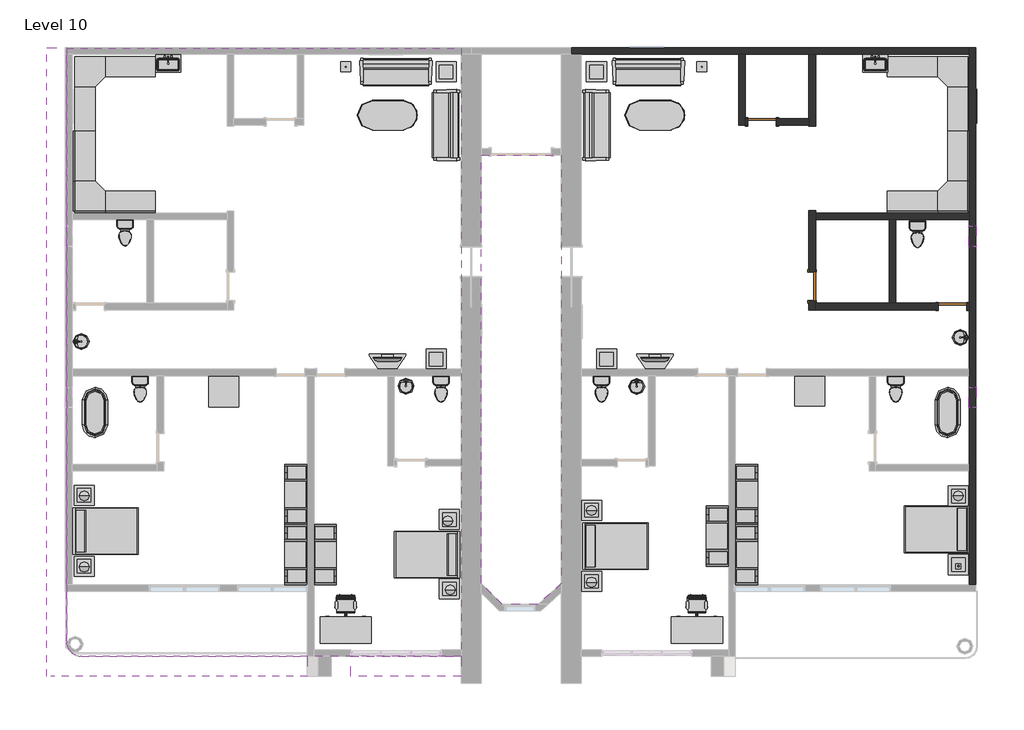
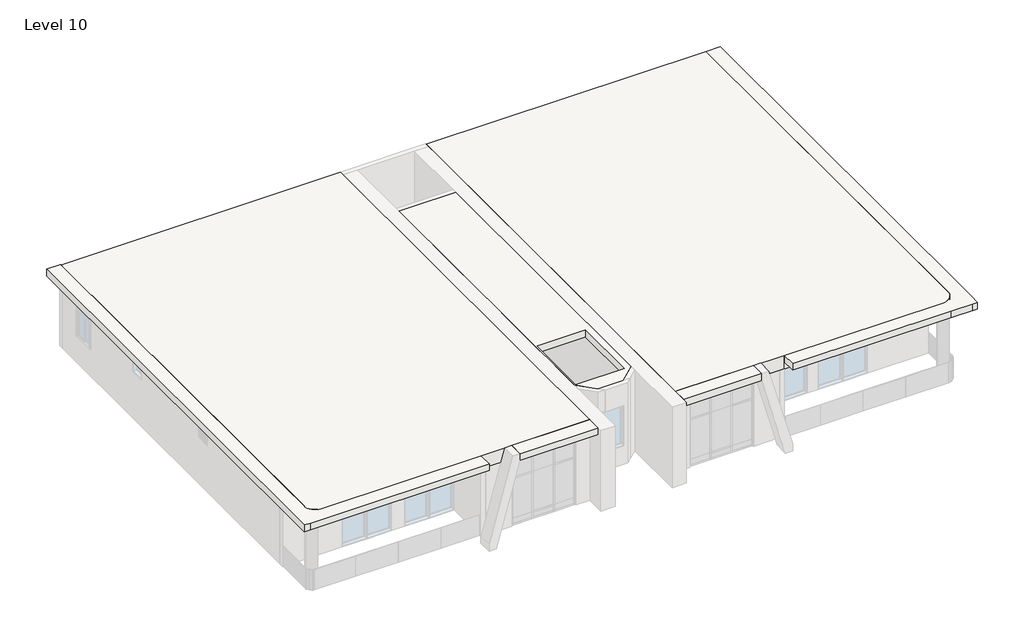
# One storey, part 3 of 3: 42 furniture elements, 14 flow terminals, 10 light fixtures, 9 walls, 4 slabs, 3 doors, 3 windows.
"""IFC4 building model written with IfcOpenShell, lengths in millimetres."""

from ifc_helpers import new_model, si_unit, point, frame, frame_2d, origin, place, context, project, spatial, polyline, circle_curve, trimmed, segment, composite_curve, outline, extrude, faceted_brep, transform, mapped, element, save
from components import door_2703ae13, door_10fd3a06, flow_terminal_38af2918, flow_terminal_d49f872f, toilet_domestic_3d_toilet_domestic_3d_f7549cf7, toilet_domestic_3d_toilet_domestic_3d_183bbd19, flow_terminal_b374fae2, furniture_07436f11, furniture_096e7f55, chair_task_arms_chair_task_arms_fa5a08ef, furniture_072f6425, furniture_cf0b6580, furniture_aff9b2fb, furniture_56245f3a, tv_stand_tv_stand_6ce107e5, furniture_b5c51a22, furniture_2c34a4f9, furniture_4d44e21c, furniture_45e3acac, light_fixture_100w_120v_8564026f, table_lamp_hemispheric_60w_120v_02721d88, window_0038ecf3, window_54100e87

model = new_model("IFC4")

# Units and contexts
model_context = context("Model", 3, world=origin())
ifc_project = project(units=[si_unit("LENGTHUNIT", "METRE", prefix="MILLI")], contexts=[model_context])

# Site, building, storey
site = spatial("IfcSite", under=ifc_project)
building = spatial("IfcBuilding", under=site)
storey = spatial("IfcBuildingStorey", under=building, Name="Level 10", Elevation=32918.4)

# Doors
placement = place(None, origin())
door_shape = door_2703ae13(model_context)
element("IfcDoor", 1, ObjectType="Door-Single-Panel.0001 : 34\" x 80\"", at=placement, inside=storey, context=model_context, shape_type="MappedRepresentation", body=[
    mapped(door_shape, transform((2522.0012296, 9464.0758558, 32918.4), x_axis=(-1.0, 0.0, 0.0), y_axis=(0.0, -1.0, 0.0), z_axis=(0.0, 0.0, 1.0))),
])
door_2_shape = door_10fd3a06(model_context)
element("IfcDoor", 2, ObjectType="Door-Single-Panel.0001 : 34\" x 80\"", at=placement, inside=storey, context=model_context, shape_type="MappedRepresentation", body=[
    mapped(door_2_shape, transform((8313.2012296, 3850.6758558, 32918.4), x_axis=(1.0, 0.0, 0.0), y_axis=(0.0, 1.0, 0.0), z_axis=(0.0, 0.0, 1.0))),
])
element("IfcDoor", 3, ObjectType="Door-Single-Panel.0001 : 34\" x 80\"", at=placement, inside=storey, context=model_context, shape_type="MappedRepresentation", body=[
    mapped(door_2_shape, transform((4046.0012296, 4460.2758558, 32918.4), x_axis=(0.0, -1.0, 0.0), y_axis=(1.0, 0.0, 0.0), z_axis=(0.0, 0.0, 1.0))),
])

# Flow terminals
flow_terminal_shape = flow_terminal_38af2918(model_context)
element("IfcFlowTerminal", 4, ObjectType="Sink Kitchen-Single : 30\" x 21\"", at=placement, inside=storey, context=model_context, shape_type="MappedRepresentation", body=[
    mapped(flow_terminal_shape, transform((-15540.388011, 11239.7304546, 32918.4), x_axis=(1.0, 0.0, 0.0), y_axis=(0.0, 1.0, 0.0), z_axis=(0.0, 0.0, 1.0))),
])
element("IfcFlowTerminal", 5, ObjectType="Sink Kitchen-Single : 30\" x 21\"", at=placement, inside=storey, context=model_context, shape_type="MappedRepresentation", body=[
    mapped(flow_terminal_shape, transform((5948.011989, 11239.7304546, 32918.4), x_axis=(1.0, 0.0, 0.0), y_axis=(0.0, 1.0, 0.0), z_axis=(0.0, 0.0, 1.0))),
])
flow_terminal_2_shape = flow_terminal_d49f872f(model_context)
element("IfcFlowTerminal", 6, ObjectType="Sink Vanity-Round : 19\" x 19\"", at=placement, inside=storey, context=model_context, shape_type="MappedRepresentation", body=[
    mapped(flow_terminal_2_shape, transform((-18084.6070794, 2687.2241152, 32918.4), x_axis=(0.0, 1.0, 0.0), y_axis=(-1.0, 0.0, 0.0), z_axis=(0.0, 0.0, 1.0))),
])
element("IfcFlowTerminal", 7, ObjectType="Sink Vanity-Round : 19\" x 19\"", at=placement, inside=storey, context=model_context, shape_type="MappedRepresentation", body=[
    mapped(flow_terminal_2_shape, transform((8462.2249463, 3007.5275963, 32918.4), x_axis=(0.0, -1.0, 0.0), y_axis=(1.0, 0.0, 0.0), z_axis=(0.0, 0.0, 1.0))),
])
element("IfcFlowTerminal", 8, ObjectType="Sink Vanity-Round : 19\" x 19\"", at=placement, inside=storey, context=model_context, shape_type="MappedRepresentation", body=[
    mapped(flow_terminal_2_shape, transform((-8395.050511, 1341.8921141, 32918.4), x_axis=(1.0, 0.0, 0.0), y_axis=(0.0, 1.0, 0.0), z_axis=(0.0, 0.0, 1.0))),
])
element("IfcFlowTerminal", 9, ObjectType="Sink Vanity-Round : 19\" x 19\"", at=placement, inside=storey, context=model_context, shape_type="MappedRepresentation", body=[
    mapped(flow_terminal_2_shape, transform((-1384.650511, 1331.0855344, 32918.4), x_axis=(1.0, 0.0, 0.0), y_axis=(0.0, 1.0, 0.0), z_axis=(0.0, 0.0, 1.0))),
])
toilet_domestic_3d_toilet_domestic_3d_shape = toilet_domestic_3d_toilet_domestic_3d_f7549cf7(model_context)
toilet_domestic_3d_toilet_domestic_3d_2_shape = toilet_domestic_3d_toilet_domestic_3d_183bbd19(model_context)
element("IfcFlowTerminal", 10, ObjectType="Toilet-Domestic-3D : Toilet-Domestic-3D", at=placement, inside=storey, context=model_context, shape_type="MappedRepresentation", body=[
    mapped(toilet_domestic_3d_toilet_domestic_3d_shape, transform((6586.0012296, 1247.7798284, 32918.4), x_axis=(1.0, 0.0, 0.0), y_axis=(0.0, 1.0, 0.0), z_axis=(0.0, 0.0, 1.0))),
    mapped(toilet_domestic_3d_toilet_domestic_3d_2_shape, transform((6586.0012296, 1247.7798284, 32918.4), x_axis=(1.0, 0.0, 0.0), y_axis=(0.0, 1.0, 0.0), z_axis=(0.0, 0.0, 1.0))),
])
element("IfcFlowTerminal", 11, ObjectType="Toilet-Domestic-3D : Toilet-Domestic-3D", at=placement, inside=storey, context=model_context, shape_type="MappedRepresentation", body=[
    mapped(toilet_domestic_3d_toilet_domestic_3d_shape, transform((-2354.7987704, 1247.7798284, 32918.4), x_axis=(1.0, 0.0, 0.0), y_axis=(0.0, 1.0, 0.0), z_axis=(0.0, 0.0, 1.0))),
    mapped(toilet_domestic_3d_toilet_domestic_3d_2_shape, transform((-2354.7987704, 1247.7798284, 32918.4), x_axis=(1.0, 0.0, 0.0), y_axis=(0.0, 1.0, 0.0), z_axis=(0.0, 0.0, 1.0))),
])
element("IfcFlowTerminal", 12, ObjectType="Toilet-Domestic-3D : Toilet-Domestic-3D", at=placement, inside=storey, context=model_context, shape_type="MappedRepresentation", body=[
    mapped(toilet_domestic_3d_toilet_domestic_3d_shape, transform((-16375.5987704, 1247.7798284, 32918.4), x_axis=(1.0, 0.0, 0.0), y_axis=(0.0, 1.0, 0.0), z_axis=(0.0, 0.0, 1.0))),
    mapped(toilet_domestic_3d_toilet_domestic_3d_2_shape, transform((-16375.5987704, 1247.7798284, 32918.4), x_axis=(1.0, 0.0, 0.0), y_axis=(0.0, 1.0, 0.0), z_axis=(0.0, 0.0, 1.0))),
])
element("IfcFlowTerminal", 13, ObjectType="Toilet-Domestic-3D : Toilet-Domestic-3D", at=placement, inside=storey, context=model_context, shape_type="MappedRepresentation", body=[
    mapped(toilet_domestic_3d_toilet_domestic_3d_shape, transform((-16832.7987704, 5997.5798284, 32918.4), x_axis=(1.0, 0.0, 0.0), y_axis=(0.0, 1.0, 0.0), z_axis=(0.0, 0.0, 1.0))),
    mapped(toilet_domestic_3d_toilet_domestic_3d_2_shape, transform((-16832.7987704, 5997.5798284, 32918.4), x_axis=(1.0, 0.0, 0.0), y_axis=(0.0, 1.0, 0.0), z_axis=(0.0, 0.0, 1.0))),
])
element("IfcFlowTerminal", 14, ObjectType="Toilet-Domestic-3D : Toilet-Domestic-3D", at=placement, inside=storey, context=model_context, shape_type="MappedRepresentation", body=[
    mapped(toilet_domestic_3d_toilet_domestic_3d_shape, transform((7246.4012296, 5946.7798284, 32918.4), x_axis=(1.0, 0.0, 0.0), y_axis=(0.0, 1.0, 0.0), z_axis=(0.0, 0.0, 1.0))),
    mapped(toilet_domestic_3d_toilet_domestic_3d_2_shape, transform((7246.4012296, 5946.7798284, 32918.4), x_axis=(1.0, 0.0, 0.0), y_axis=(0.0, 1.0, 0.0), z_axis=(0.0, 0.0, 1.0))),
])
element("IfcFlowTerminal", 15, ObjectType="Toilet-Domestic-3D : Toilet-Domestic-3D", at=placement, inside=storey, context=model_context, shape_type="MappedRepresentation", body=[
    mapped(toilet_domestic_3d_toilet_domestic_3d_shape, transform((-7231.5987704, 1247.7798284, 32918.4), x_axis=(1.0, 0.0, 0.0), y_axis=(0.0, 1.0, 0.0), z_axis=(0.0, 0.0, 1.0))),
    mapped(toilet_domestic_3d_toilet_domestic_3d_2_shape, transform((-7231.5987704, 1247.7798284, 32918.4), x_axis=(1.0, 0.0, 0.0), y_axis=(0.0, 1.0, 0.0), z_axis=(0.0, 0.0, 1.0))),
])
flow_terminal_3_shape = flow_terminal_b374fae2(model_context)
element("IfcFlowTerminal", 16, ObjectType="Tub-Free Standing-3D : 30\" x 60\"", at=placement, inside=storey, context=model_context, shape_type="MappedRepresentation", body=[
    mapped(flow_terminal_3_shape, transform((-17747.1987704, 624.8758558, 32918.4), x_axis=(1.0, 0.0, 0.0), y_axis=(0.0, 1.0, 0.0), z_axis=(0.0, 0.0, 1.0))),
])
element("IfcFlowTerminal", 17, ObjectType="Tub-Free Standing-3D : 30\" x 60\"", at=placement, inside=storey, context=model_context, shape_type="MappedRepresentation", body=[
    mapped(flow_terminal_3_shape, transform((8160.8012296, 624.8758558, 32918.4), x_axis=(1.0, 0.0, 0.0), y_axis=(0.0, 1.0, 0.0), z_axis=(0.0, 0.0, 1.0))),
])

# Furniture
furniture_shape = furniture_07436f11(model_context)
element("IfcFurniture", 18, ObjectType="96\" x 96\"", at=placement, inside=storey, context=model_context, shape_type="MappedRepresentation", body=[
    mapped(furniture_shape, transform((-18275.8670182, 11991.0988634, 32918.4), x_axis=(1.0, 0.0, 0.0), y_axis=(0.0, 1.0, 0.0), z_axis=(0.0, 0.0, 1.0))),
])
element("IfcFurniture", 19, ObjectType="96\" x 96\"", at=placement, inside=storey, context=model_context, shape_type="MappedRepresentation", body=[
    mapped(furniture_shape, transform((9316.2242372, 11364.3441035, 32918.4), x_axis=(0.0, -1.0, 0.0), y_axis=(1.0, 0.0, 0.0), z_axis=(0.0, 0.0, 1.0))),
])
furniture_2_shape = furniture_096e7f55(model_context)
element("IfcFurniture", 20, ObjectType="Bed-Shaker : Double 56\" x 78\"", at=placement, inside=storey, context=model_context, shape_type="MappedRepresentation", body=[
    mapped(furniture_2_shape, transform((-18407.5987704, -2962.8741442, 32918.4), x_axis=(0.0, 1.0, 0.0), y_axis=(-1.0, 0.0, 0.0), z_axis=(0.0, 0.0, 1.0))),
])
element("IfcFurniture", 21, ObjectType="Bed-Shaker : Double 56\" x 78\"", at=placement, inside=storey, context=model_context, shape_type="MappedRepresentation", body=[
    mapped(furniture_2_shape, transform((-6672.7987704, -3712.1741442, 32918.4), x_axis=(0.0, -1.0, 0.0), y_axis=(1.0, 0.0, 0.0), z_axis=(0.0, 0.0, 1.0))),
])
element("IfcFurniture", 22, ObjectType="Bed-Shaker : Double 56\" x 78\"", at=placement, inside=storey, context=model_context, shape_type="MappedRepresentation", body=[
    mapped(furniture_2_shape, transform((-2913.5987704, -3420.0741442, 32918.4), x_axis=(0.0, 1.0, 0.0), y_axis=(-1.0, 0.0, 0.0), z_axis=(0.0, 0.0, 1.0))),
])
element("IfcFurniture", 23, ObjectType="Bed-Shaker : Double 56\" x 78\"", at=placement, inside=storey, context=model_context, shape_type="MappedRepresentation", body=[
    mapped(furniture_2_shape, transform((8821.2012296, -2950.1741442, 32918.4), x_axis=(0.0, -1.0, 0.0), y_axis=(1.0, 0.0, 0.0), z_axis=(0.0, 0.0, 1.0))),
])
chair_task_arms_chair_task_arms_shape = chair_task_arms_chair_task_arms_fa5a08ef(model_context)
element("IfcFurniture", 24, ObjectType="Chair-Task Arms : Chair-Task Arms", at=placement, inside=storey, context=model_context, shape_type="MappedRepresentation", body=[
    mapped(chair_task_arms_chair_task_arms_shape, transform((681.7920493, -5184.3566833, 32918.4), x_axis=(-1.0, 0.0, 0.0), y_axis=(0.0, -1.0, 0.0), z_axis=(0.0, 0.0, 1.0))),
])
element("IfcFurniture", 25, ObjectType="Chair-Task Arms : Chair-Task Arms", at=placement, inside=storey, context=model_context, shape_type="MappedRepresentation", body=[
    mapped(chair_task_arms_chair_task_arms_shape, transform((-9986.2079507, -5184.3566833, 32918.4), x_axis=(-1.0, 0.0, 0.0), y_axis=(0.0, -1.0, 0.0), z_axis=(0.0, 0.0, 1.0))),
])
furniture_3_shape = furniture_072f6425(model_context)
element("IfcFurniture", 26, ObjectType="Desk : 60\" x 30\"", at=placement, inside=storey, context=model_context, shape_type="MappedRepresentation", body=[
    mapped(furniture_3_shape, transform((-10889.1987704, -6371.702585, 32918.4), x_axis=(1.0, 0.0, 0.0), y_axis=(0.0, 1.0, 0.0), z_axis=(0.0, 0.0, 1.0))),
])
element("IfcFurniture", 27, ObjectType="Desk : 60\" x 30\"", at=placement, inside=storey, context=model_context, shape_type="MappedRepresentation", body=[
    mapped(furniture_3_shape, transform((-221.1987704, -6371.702585, 32918.4), x_axis=(1.0, 0.0, 0.0), y_axis=(0.0, 1.0, 0.0), z_axis=(0.0, 0.0, 1.0))),
])
furniture_4_shape = furniture_cf0b6580(model_context)
element("IfcFurniture", 28, ObjectType="Entertainment Center : 72\" x 72\" x 24\"", at=placement, inside=storey, context=model_context, shape_type="MappedRepresentation", body=[
    mapped(furniture_4_shape, transform((1607.6012296, -3134.3241442, 32918.4), x_axis=(0.0, -1.0, 0.0), y_axis=(1.0, 0.0, 0.0), z_axis=(0.0, 0.0, 1.0))),
])
element("IfcFurniture", 29, ObjectType="Entertainment Center : 72\" x 72\" x 24\"", at=placement, inside=storey, context=model_context, shape_type="MappedRepresentation", body=[
    mapped(furniture_4_shape, transform((1607.6012296, -3693.1241442, 32918.4), x_axis=(0.0, 1.0, 0.0), y_axis=(-1.0, 0.0, 0.0), z_axis=(0.0, 0.0, 1.0))),
])
element("IfcFurniture", 30, ObjectType="Entertainment Center : 72\" x 72\" x 24\"", at=placement, inside=storey, context=model_context, shape_type="MappedRepresentation", body=[
    mapped(furniture_4_shape, transform((1607.6012296, -1864.3241442, 32918.4), x_axis=(0.0, 1.0, 0.0), y_axis=(-1.0, 0.0, 0.0), z_axis=(0.0, 0.0, 1.0))),
])
element("IfcFurniture", 31, ObjectType="Entertainment Center : 72\" x 72\" x 24\"", at=placement, inside=storey, context=model_context, shape_type="MappedRepresentation", body=[
    mapped(furniture_4_shape, transform((-11193.9987704, -3693.1241442, 32918.4), x_axis=(0.0, -1.0, 0.0), y_axis=(1.0, 0.0, 0.0), z_axis=(0.0, 0.0, 1.0))),
])
element("IfcFurniture", 32, ObjectType="Entertainment Center : 72\" x 72\" x 24\"", at=placement, inside=storey, context=model_context, shape_type="MappedRepresentation", body=[
    mapped(furniture_4_shape, transform((-11193.9987704, -1864.3241442, 32918.4), x_axis=(0.0, -1.0, 0.0), y_axis=(1.0, 0.0, 0.0), z_axis=(0.0, 0.0, 1.0))),
])
element("IfcFurniture", 33, ObjectType="Entertainment Center : 72\" x 72\" x 24\"", at=placement, inside=storey, context=model_context, shape_type="MappedRepresentation", body=[
    mapped(furniture_4_shape, transform((-11193.9987704, -3693.1241442, 32918.4), x_axis=(0.0, 1.0, 0.0), y_axis=(-1.0, 0.0, 0.0), z_axis=(0.0, 0.0, 1.0))),
])
furniture_5_shape = furniture_aff9b2fb(model_context)
element("IfcFurniture", 34, ObjectType="Sofa-Pensi : 84\"", at=placement, inside=storey, context=model_context, shape_type="MappedRepresentation", body=[
    mapped(furniture_5_shape, transform((-8881.8050204, 10710.9660197, 32918.4), x_axis=(1.0, 0.0, 0.0), y_axis=(0.0, 1.0, 0.0), z_axis=(0.0, 0.0, 1.0))),
])
element("IfcFurniture", 35, ObjectType="Sofa-Pensi : 84\"", at=placement, inside=storey, context=model_context, shape_type="MappedRepresentation", body=[
    mapped(furniture_5_shape, transform((-7356.3086065, 9641.0821058, 32918.4), x_axis=(0.0, -1.0, 0.0), y_axis=(1.0, 0.0, 0.0), z_axis=(0.0, 0.0, 1.0))),
])
element("IfcFurniture", 36, ObjectType="Sofa-Pensi : 84\"", at=placement, inside=storey, context=model_context, shape_type="MappedRepresentation", body=[
    mapped(furniture_5_shape, transform((-2230.0889343, 9083.8696058, 32918.4), x_axis=(0.0, 1.0, 0.0), y_axis=(-1.0, 0.0, 0.0), z_axis=(0.0, 0.0, 1.0))),
])
element("IfcFurniture", 37, ObjectType="Sofa-Pensi : 84\"", at=placement, inside=storey, context=model_context, shape_type="MappedRepresentation", body=[
    mapped(furniture_5_shape, transform((-1211.0050204, 10710.9660197, 32918.4), x_axis=(1.0, 0.0, 0.0), y_axis=(0.0, 1.0, 0.0), z_axis=(0.0, 0.0, 1.0))),
])
furniture_6_shape = furniture_56245f3a(model_context)
element("IfcFurniture", 38, ObjectType="TV - Flat Screen : 32\"", at=placement, inside=storey, context=model_context, shape_type="MappedRepresentation", body=[
    mapped(furniture_6_shape, transform((-8861.1432846, 2232.8144794, 33832.8), x_axis=(-1.0, 0.0, 0.0), y_axis=(0.0, -1.0, 0.0), z_axis=(0.0, 0.0, 1.0))),
])
element("IfcFurniture", 39, ObjectType="TV - Flat Screen : 32\"", at=placement, inside=storey, context=model_context, shape_type="MappedRepresentation", body=[
    mapped(furniture_6_shape, transform((-733.1432846, 2232.8144794, 33832.8), x_axis=(-1.0, 0.0, 0.0), y_axis=(0.0, -1.0, 0.0), z_axis=(0.0, 0.0, 1.0))),
])
tv_stand_tv_stand_shape = tv_stand_tv_stand_6ce107e5(model_context)
element("IfcFurniture", 40, ObjectType="TV Stand : TV Stand", at=placement, inside=storey, context=model_context, shape_type="MappedRepresentation", body=[
    mapped(tv_stand_tv_stand_shape, transform((-8732.0107683, 1945.6758558, 32918.4), x_axis=(-1.0, 0.0, 0.0), y_axis=(0.0, -1.0, 0.0), z_axis=(0.0, 0.0, 1.0))),
])
element("IfcFurniture", 41, ObjectType="TV Stand : TV Stand", at=placement, inside=storey, context=model_context, shape_type="MappedRepresentation", body=[
    mapped(tv_stand_tv_stand_shape, transform((-604.0107683, 1945.6758558, 32918.4), x_axis=(-1.0, 0.0, 0.0), y_axis=(0.0, -1.0, 0.0), z_axis=(0.0, 0.0, 1.0))),
])
furniture_7_shape = furniture_b5c51a22(model_context)
element("IfcFurniture", 42, ObjectType="Table-Coffee : 24\" x 24\" x 24\"", at=placement, inside=storey, context=model_context, shape_type="MappedRepresentation", body=[
    mapped(furniture_7_shape, transform((-7097.4645371, 10892.864778, 32918.4), x_axis=(1.0, 0.0, 0.0), y_axis=(0.0, 1.0, 0.0), z_axis=(0.0, 0.0, 1.0))),
])
element("IfcFurniture", 43, ObjectType="Table-Coffee : 24\" x 24\" x 24\"", at=placement, inside=storey, context=model_context, shape_type="MappedRepresentation", body=[
    mapped(furniture_7_shape, transform((-2525.4645371, 10892.864778, 32918.4), x_axis=(1.0, 0.0, 0.0), y_axis=(0.0, 1.0, 0.0), z_axis=(0.0, 0.0, 1.0))),
])
element("IfcFurniture", 44, ObjectType="Table-Coffee : 24\" x 24\" x 24\"", at=placement, inside=storey, context=model_context, shape_type="MappedRepresentation", body=[
    mapped(furniture_7_shape, transform((-7402.2645371, 2155.264778, 32918.4), x_axis=(1.0, 0.0, 0.0), y_axis=(0.0, 1.0, 0.0), z_axis=(0.0, 0.0, 1.0))),
])
element("IfcFurniture", 45, ObjectType="Table-Coffee : 24\" x 24\" x 24\"", at=placement, inside=storey, context=model_context, shape_type="MappedRepresentation", body=[
    mapped(furniture_7_shape, transform((-2220.6645371, 2155.264778, 32918.4), x_axis=(1.0, 0.0, 0.0), y_axis=(0.0, 1.0, 0.0), z_axis=(0.0, 0.0, 1.0))),
])
element("IfcFurniture", 46, ObjectType="Table-Coffee : 24\" x 24\" x 24\"", at=placement, inside=storey, context=model_context, shape_type="MappedRepresentation", body=[
    mapped(furniture_7_shape, transform((-2677.8645371, -4601.135222, 32918.4), x_axis=(1.0, 0.0, 0.0), y_axis=(0.0, 1.0, 0.0), z_axis=(0.0, 0.0, 1.0))),
])
element("IfcFurniture", 47, ObjectType="Table-Coffee : 24\" x 24\" x 24\"", at=placement, inside=storey, context=model_context, shape_type="MappedRepresentation", body=[
    mapped(furniture_7_shape, transform((-18095.6645371, -4143.935222, 32918.4), x_axis=(1.0, 0.0, 0.0), y_axis=(0.0, 1.0, 0.0), z_axis=(0.0, 0.0, 1.0))),
])
element("IfcFurniture", 48, ObjectType="Table-Coffee : 24\" x 24\" x 24\"", at=placement, inside=storey, context=model_context, shape_type="MappedRepresentation", body=[
    mapped(furniture_7_shape, transform((-18095.6645371, -1984.935222, 32918.4), x_axis=(1.0, 0.0, 0.0), y_axis=(0.0, 1.0, 0.0), z_axis=(0.0, 0.0, 1.0))),
])
element("IfcFurniture", 49, ObjectType="Table-Coffee : 24\" x 24\" x 24\"", at=placement, inside=storey, context=model_context, shape_type="MappedRepresentation", body=[
    mapped(furniture_7_shape, transform((-2677.8645371, -2442.135222, 32918.4), x_axis=(1.0, 0.0, 0.0), y_axis=(0.0, 1.0, 0.0), z_axis=(0.0, 0.0, 1.0))),
])
element("IfcFurniture", 50, ObjectType="Table-Coffee : 24\" x 24\" x 24\"", at=placement, inside=storey, context=model_context, shape_type="MappedRepresentation", body=[
    mapped(furniture_7_shape, transform((8472.7354629, -4093.135222, 32918.4), x_axis=(1.0, 0.0, 0.0), y_axis=(0.0, 1.0, 0.0), z_axis=(0.0, 0.0, 1.0))),
])
element("IfcFurniture", 51, ObjectType="Table-Coffee : 24\" x 24\" x 24\"", at=placement, inside=storey, context=model_context, shape_type="MappedRepresentation", body=[
    mapped(furniture_7_shape, transform((8472.7354629, -2010.335222, 32918.4), x_axis=(1.0, 0.0, 0.0), y_axis=(0.0, 1.0, 0.0), z_axis=(0.0, 0.0, 1.0))),
])
element("IfcFurniture", 52, ObjectType="Table-Coffee : 24\" x 24\" x 24\"", at=placement, inside=storey, context=model_context, shape_type="MappedRepresentation", body=[
    mapped(furniture_7_shape, transform((-6995.8645371, -4832.0414601, 32918.4), x_axis=(1.0, 0.0, 0.0), y_axis=(0.0, 1.0, 0.0), z_axis=(0.0, 0.0, 1.0))),
])
element("IfcFurniture", 53, ObjectType="Table-Coffee : 24\" x 24\" x 24\"", at=placement, inside=storey, context=model_context, shape_type="MappedRepresentation", body=[
    mapped(furniture_7_shape, transform((-6995.8645371, -2723.8414601, 32918.4), x_axis=(1.0, 0.0, 0.0), y_axis=(0.0, 1.0, 0.0), z_axis=(0.0, 0.0, 1.0))),
])
furniture_8_shape = furniture_2c34a4f9(model_context)
element("IfcFurniture", 54, ObjectType="Table-Dining Oval : 36\" x 72\"", at=placement, inside=storey, context=model_context, shape_type="MappedRepresentation", body=[
    mapped(furniture_8_shape, transform((-8455.3790983, 10025.3742164, 32918.4), x_axis=(1.0, 0.0, 0.0), y_axis=(0.0, 1.0, 0.0), z_axis=(0.0, 0.0, 1.0))),
])
element("IfcFurniture", 55, ObjectType="Table-Dining Oval : 36\" x 72\"", at=placement, inside=storey, context=model_context, shape_type="MappedRepresentation", body=[
    mapped(furniture_8_shape, transform((-327.3790983, 10025.3742164, 32918.4), x_axis=(1.0, 0.0, 0.0), y_axis=(0.0, 1.0, 0.0), z_axis=(0.0, 0.0, 1.0))),
])
furniture_9_shape = furniture_4d44e21c(model_context)
element("IfcFurniture", 56, ObjectType="Table-Rectangular : 36\" x 36\"", at=placement, inside=storey, context=model_context, shape_type="MappedRepresentation", body=[
    mapped(furniture_9_shape, transform((-13835.5987704, 1259.8758558, 32918.4), x_axis=(1.0, 0.0, 0.0), y_axis=(0.0, 1.0, 0.0), z_axis=(0.0, 0.0, 1.0))),
])
element("IfcFurniture", 57, ObjectType="Table-Rectangular : 36\" x 36\"", at=placement, inside=storey, context=model_context, shape_type="MappedRepresentation", body=[
    mapped(furniture_9_shape, transform((3969.8012296, 1285.2758558, 32918.4), x_axis=(1.0, 0.0, 0.0), y_axis=(0.0, 1.0, 0.0), z_axis=(0.0, 0.0, 1.0))),
])
furniture_10_shape = furniture_45e3acac(model_context)
element("IfcFurniture", 58, ObjectType="Work Station Cubicle : 96\" x 96\"", at=placement, inside=storey, context=model_context, shape_type="MappedRepresentation", body=[
    mapped(furniture_10_shape, transform((-18902.621778, 6827.207608, 32918.4), x_axis=(0.0, 1.0, 0.0), y_axis=(-1.0, 0.0, 0.0), z_axis=(0.0, 0.0, 1.0))),
])
element("IfcFurniture", 59, ObjectType="Work Station Cubicle : 96\" x 96\"", at=placement, inside=storey, context=model_context, shape_type="MappedRepresentation", body=[
    mapped(furniture_10_shape, transform((8689.4694774, 6200.4528481, 32918.4), x_axis=(-1.0, 0.0, 0.0), y_axis=(0.0, -1.0, 0.0), z_axis=(0.0, 0.0, 1.0))),
])

# Light fixtures
light_fixture_100w_120v_shape = light_fixture_100w_120v_8564026f(model_context)
element("IfcLightFixture", 60, ObjectType="100W - 120V", at=placement, inside=storey, context=model_context, shape_type="MappedRepresentation", body=[
    mapped(light_fixture_100w_120v_shape, transform((-10127.1987704, 11140.4758558, 32918.4), x_axis=(1.0, 0.0, 0.0), y_axis=(0.0, 1.0, 0.0), z_axis=(0.0, 0.0, 1.0))),
])
element("IfcLightFixture", 61, ObjectType="100W - 120V", at=placement, inside=storey, context=model_context, shape_type="MappedRepresentation", body=[
    mapped(light_fixture_100w_120v_shape, transform((693.2012296, 11140.4758558, 32918.4), x_axis=(1.0, 0.0, 0.0), y_axis=(0.0, 1.0, 0.0), z_axis=(0.0, 0.0, 1.0))),
])
table_lamp_hemispheric_60w_120v_shape = table_lamp_hemispheric_60w_120v_02721d88(model_context)
element("IfcLightFixture", 62, ObjectType="Table Lamp - Hemispheric : 60W - 120V", at=placement, inside=storey, context=model_context, shape_type="MappedRepresentation", body=[
    mapped(table_lamp_hemispheric_60w_120v_shape, transform((-18077.3987704, -1915.1241442, 33528.0), x_axis=(1.0, 0.0, 0.0), y_axis=(0.0, 1.0, 0.0), z_axis=(0.0, 0.0, 1.0))),
])
element("IfcLightFixture", 63, ObjectType="Table Lamp - Hemispheric : 60W - 120V", at=placement, inside=storey, context=model_context, shape_type="MappedRepresentation", body=[
    mapped(table_lamp_hemispheric_60w_120v_shape, transform((-7028.3987704, -2666.7303823, 33528.0), x_axis=(1.0, 0.0, 0.0), y_axis=(0.0, 1.0, 0.0), z_axis=(0.0, 0.0, 1.0))),
])
element("IfcLightFixture", 64, ObjectType="Table Lamp - Hemispheric : 60W - 120V", at=placement, inside=storey, context=model_context, shape_type="MappedRepresentation", body=[
    mapped(table_lamp_hemispheric_60w_120v_shape, transform((-2659.5987704, -2346.9241442, 33528.0), x_axis=(1.0, 0.0, 0.0), y_axis=(0.0, 1.0, 0.0), z_axis=(0.0, 0.0, 1.0))),
])
element("IfcLightFixture", 65, ObjectType="Table Lamp - Hemispheric : 60W - 120V", at=placement, inside=storey, context=model_context, shape_type="MappedRepresentation", body=[
    mapped(table_lamp_hemispheric_60w_120v_shape, transform((8491.0012296, -4048.7241442, 33832.8), x_axis=(1.0, 0.0, 0.0), y_axis=(0.0, 1.0, 0.0), z_axis=(0.0, 0.0, 1.0))),
])
element("IfcLightFixture", 66, ObjectType="Table Lamp - Hemispheric : 60W - 120V", at=placement, inside=storey, context=model_context, shape_type="MappedRepresentation", body=[
    mapped(table_lamp_hemispheric_60w_120v_shape, transform((8491.0012296, -1915.1241442, 33528.0), x_axis=(1.0, 0.0, 0.0), y_axis=(0.0, 1.0, 0.0), z_axis=(0.0, 0.0, 1.0))),
])
element("IfcLightFixture", 67, ObjectType="Table Lamp - Hemispheric : 60W - 120V", at=placement, inside=storey, context=model_context, shape_type="MappedRepresentation", body=[
    mapped(table_lamp_hemispheric_60w_120v_shape, transform((-2659.5987704, -4531.3241442, 33528.0), x_axis=(1.0, 0.0, 0.0), y_axis=(0.0, 1.0, 0.0), z_axis=(0.0, 0.0, 1.0))),
])
element("IfcLightFixture", 68, ObjectType="Table Lamp - Hemispheric : 60W - 120V", at=placement, inside=storey, context=model_context, shape_type="MappedRepresentation", body=[
    mapped(table_lamp_hemispheric_60w_120v_shape, transform((-6952.1987704, -4762.2303823, 33528.0), x_axis=(1.0, 0.0, 0.0), y_axis=(0.0, 1.0, 0.0), z_axis=(0.0, 0.0, 1.0))),
])
element("IfcLightFixture", 69, ObjectType="Table Lamp - Hemispheric : 60W - 120V", at=placement, inside=storey, context=model_context, shape_type="MappedRepresentation", body=[
    mapped(table_lamp_hemispheric_60w_120v_shape, transform((-18077.3987704, -4074.1241442, 33528.0), x_axis=(1.0, 0.0, 0.0), y_axis=(0.0, 1.0, 0.0), z_axis=(0.0, 0.0, 1.0))),
])

# Slabs
element("IfcSlab", 70, ObjectType="Generic - 12\" cream", at=placement, inside=storey, context=model_context, shape_type="SweptSolid", body=[
    extrude(outline(composite_curve([segment(polyline([(-6621.9987704, 11699.2758558), (-6621.9987704, -6791.9241442), (-11295.5987704, -6791.9241442), (-18153.5987704, -6791.9241442)]), True, "CONTINUOUS"), segment(trimmed(circle_curve(frame_2d((-18153.5987704, -6334.7241442)), 457.2), [point((-18153.5987704, -6791.9241442))], [point((-18610.7987704, -6334.7241442))], False, "CARTESIAN"), True, "CONTINUOUS"), segment(polyline([(-18610.7987704, -6334.7241442), (-18610.7987704, 11699.2758558), (-6621.9987704, 11699.2758558)]), True, "CONTINUOUS")], self_intersect=False)), frame((0.0, 0.0, 35966.4), z_axis=(0.0, 0.0, 1.0), x_axis=(1.0, 0.0, 0.0)), (0.0, 0.0, 1.0), 609.6),
    extrude(outline(composite_curve([segment(trimmed(circle_curve(frame_2d((8511.8043381, -6277.3874522)), 514.536692), [point((9024.4012296, -6322.0241442))], [point((8511.8043381, -6791.9241442))], False, "CARTESIAN"), True, "CONTINUOUS"), segment(polyline([(8511.8043381, -6791.9241442), (1709.2012296, -6791.9241442), (-2862.7987704, -6791.9241442), (-2964.3987704, -6791.9241442), (-2964.3987704, 11699.2758558), (9024.4012296, 11699.2758558), (9024.4012296, -6322.0241442)]), True, "CONTINUOUS")], self_intersect=False)), frame((0.0, 0.0, 35966.4), z_axis=(0.0, 0.0, 1.0), x_axis=(1.0, 0.0, 0.0)), (0.0, 0.0, 1.0), 609.6),
])
element("IfcSlab", 71, ObjectType="Generic - 12\" white", at=placement, inside=storey, context=model_context, shape_type="SweptSolid", body=[
    extrude(outline(composite_curve([segment(polyline([(9634.0012296, 11699.2758558), (9634.0012296, -6931.6241442), (9634.0012296, -7401.5241442), (9430.8012296, -7401.5241442), (8511.8043381, -7401.5241442), (1709.2012296, -7401.5241442), (1709.2012296, -6791.9241442), (8511.8043381, -6791.9241442)]), True, "CONTINUOUS"), segment(trimmed(circle_curve(frame_2d((8511.8043381, -6277.3874522)), 514.536692), [point((8511.8043381, -6791.9241442))], [point((9024.4012296, -6322.0241442))], True, "CARTESIAN"), True, "CONTINUOUS"), segment(polyline([(9024.4012296, -6322.0241442), (9024.4012296, 11699.2758558), (9634.0012296, 11699.2758558)]), True, "CONTINUOUS")], self_intersect=False)), frame((0.0, 0.0, 36271.2), z_axis=(0.0, 0.0, 1.0), x_axis=(1.0, 0.0, 0.0)), (0.0, 0.0, 1.0), 304.8),
    extrude(outline(composite_curve([segment(polyline([(-18610.7987704, 11724.6758558), (-18610.7987704, -6334.7241442)]), True, "CONTINUOUS"), segment(trimmed(circle_curve(frame_2d((-18153.5987704, -6334.7241442)), 457.2), [point((-18610.7987704, -6334.7241442))], [point((-18153.5987704, -6791.9241442))], True, "CARTESIAN"), True, "CONTINUOUS"), segment(polyline([(-18153.5987704, -6791.9241442), (-11295.5987704, -6791.9241442), (-11295.5987704, -7401.5241442), (-18966.3987704, -7401.5241442), (-19220.3987704, -7401.5241442), (-19220.3987704, 11724.6758558), (-18610.7987704, 11724.6758558)]), True, "CONTINUOUS")], self_intersect=False)), frame((0.0, 0.0, 36271.2), z_axis=(0.0, 0.0, 1.0), x_axis=(1.0, 0.0, 0.0)), (0.0, 0.0, 1.0), 304.8),
])
element("IfcSlab", 72, ObjectType="Generic - 12\" white", at=placement, inside=storey, context=model_context, shape_type="SweptSolid", body=[
    extrude(outline(polyline([(388.6816194, -6791.9241442), (388.6816194, -7401.5241442), (-2958.0487704, -7401.5241442), (-2958.0487704, -6791.9241442), (388.6816194, -6791.9241442)])), frame((0.0, 0.0, 36271.2), z_axis=(0.0, 0.0, 1.0), x_axis=(1.0, 0.0, 0.0)), (0.0, 0.0, 1.0), 304.8),
    extrude(outline(polyline([(-9974.7987704, -6791.9241442), (-6621.9987704, -6791.9241442), (-6621.9987704, -7401.5241442), (-9974.7987704, -7401.5241442), (-9974.7987704, -6791.9241442)])), frame((0.0, 0.0, 36271.2), z_axis=(0.0, 0.0, 1.0), x_axis=(1.0, 0.0, 0.0)), (0.0, 0.0, 1.0), 304.8),
])
element("IfcSlab", 73, ObjectType="Generic - 12\" white", at=placement, inside=storey, context=model_context, shape_type="SweptSolid", body=[
    extrude(outline(polyline([(-3573.9987704, 8448.0758558), (-3573.9987704, -1691.5549149), (-3573.9987704, -4572.9908503), (-4280.7801413, -5203.302585), (-5374.5362318, -5203.302585), (-6012.3987704, -4565.4400463), (-6012.3987704, -1691.5549149), (-6012.3987704, 8448.0758558), (-3573.9987704, 8448.0758558)]), holes=[polyline([(-5940.8822214, -4561.7549149), (-3870.7822214, -4561.7549149), (-3870.7822214, -1691.5549149), (-5940.8822214, -1691.5549149), (-5940.8822214, -4561.7549149)])]), frame((0.0, 0.0, 36271.2), z_axis=(0.0, 0.0, 1.0), x_axis=(1.0, 0.0, 0.0)), (0.0, 0.0, 1.0), 304.8),
])

# Walls
element("IfcWall", 74, ObjectType="Generic - 8\" cream", at=placement, inside=storey, context=model_context, shape_type="Brep", body=[
    faceted_brep([(8821.2012296, 11724.6758558, 32918.4), (8821.2012296, 11521.4758558, 32918.4), (8821.2012296, 6695.4758558, 32918.4), (8821.2012296, 6492.2758558, 32918.4), (8821.2012296, 3952.2758558, 32918.4), (8821.2012296, 3749.0758558, 32918.4), (8821.2012296, 1945.6758558, 32918.4), (8821.2012296, 1742.4758558, 32918.4), (8821.2012296, -949.9241442, 32918.4), (8821.2012296, -1153.1241442, 32918.4), (8821.2012296, -4607.5241442, 32918.4), (8821.2012296, -4607.5241442, 35966.4), (8821.2012296, -1153.1241442, 35966.4), (8821.2012296, -949.9241442, 35966.4), (8821.2012296, 1742.4758558, 35966.4), (8821.2012296, 1945.6758558, 35966.4), (8821.2012296, 3749.0758558, 35966.4), (8821.2012296, 3952.2758558, 35966.4), (8821.2012296, 6492.2758558, 35966.4), (8821.2012296, 6695.4758558, 35966.4), (8821.2012296, 11521.4758558, 35966.4), (8821.2012296, 11724.6758558, 35966.4), (8821.2012296, 10403.8758558, 34137.6), (8821.2012296, 10403.8758558, 35356.8), (8821.2012296, 9489.4758558, 35356.8), (8821.2012296, 9489.4758558, 34137.6), (8821.2012296, 777.2758558, 35661.6), (8821.2012296, 777.2758558, 35052.0), (8821.2012296, 1386.8758558, 35052.0), (8821.2012296, 1386.8758558, 35661.6), (8821.2012296, 6289.0758558, 35052.0), (8821.2012296, 6289.0758558, 35661.6), (8821.2012296, 5679.4758558, 35661.6), (8821.2012296, 5679.4758558, 35052.0), (9024.4012296, -4607.5241442, 32918.4), (9024.4012296, 11724.6758558, 32918.4), (9024.4012296, 11724.6758558, 35966.4), (9024.4012296, -4607.5241442, 35966.4), (9024.4012296, 10403.8758558, 35356.8), (9024.4012296, 10403.8758558, 34137.6), (9024.4012296, 9489.4758558, 34137.6), (9024.4012296, 9489.4758558, 35356.8), (9024.4012296, 777.2758558, 35052.0), (9024.4012296, 777.2758558, 35661.6), (9024.4012296, 1386.8758558, 35661.6), (9024.4012296, 1386.8758558, 35052.0), (9024.4012296, 6289.0758558, 35661.6), (9024.4012296, 6289.0758558, 35052.0), (9024.4012296, 5679.4758558, 35052.0), (9024.4012296, 5679.4758558, 35661.6)], [[[0, 1, 2, 3, 4, 5, 6, 7, 8, 9, 10, 11, 12, 13, 14, 15, 16, 17, 18, 19, 20, 21], [22, 23, 24, 25], [26, 27, 28, 29], [30, 31, 32, 33]], [[34, 35, 36, 37], [38, 39, 40, 41], [42, 43, 44, 45], [46, 47, 48, 49]], [[10, 9, 8, 7, 6, 5, 4, 3, 2, 1, 0, 35, 34]], [[21, 20, 19, 18, 17, 16, 15, 14, 13, 12, 11, 37, 36]], [[0, 21, 36, 35]], [[11, 10, 34, 37]], [[39, 38, 23, 22]], [[40, 39, 22, 25]], [[41, 40, 25, 24]], [[38, 41, 24, 23]], [[26, 43, 42, 27]], [[27, 42, 45, 28]], [[28, 45, 44, 29]], [[43, 26, 29, 44]], [[46, 31, 30, 47]], [[47, 30, 33, 48]], [[48, 33, 32, 49]], [[31, 46, 49, 32]]]),
])
element("IfcWall", 75, ObjectType="Generic - 8\" cream", at=placement, inside=storey, context=model_context, shape_type="Brep", body=[
    faceted_brep([(3944.4012296, 11521.4758558, 32918.4), (3944.4012296, 9565.6758558, 32918.4), (3944.4012296, 9362.4758558, 32918.4), (3944.4012296, 9337.0758558, 32918.4), (3944.4012296, 9337.0758558, 35966.4), (3944.4012296, 9362.4758558, 35966.4), (3944.4012296, 9565.6758558, 35966.4), (3944.4012296, 11521.4758558, 35966.4), (4147.6012296, 11521.4758558, 32918.4), (4147.6012296, 11521.4758558, 35966.4), (4147.6012296, 9337.0758558, 35966.4), (4147.6012296, 9337.0758558, 32918.4)], [[[0, 1, 2, 3, 4, 5, 6, 7]], [[8, 9, 10, 11]], [[3, 2, 1, 0, 8, 11]], [[4, 3, 11, 10]], [[7, 6, 5, 4, 10, 9]], [[0, 7, 9, 8]]]),
])
element("IfcWall", 76, ObjectType="Generic - 8\" cream", at=placement, inside=storey, context=model_context, shape_type="Brep", body=[
    faceted_brep([(4147.6012296, 6492.2758558, 32918.4), (6382.8012296, 6492.2758558, 32918.4), (6586.0012296, 6492.2758558, 32918.4), (8821.2012296, 6492.2758558, 32918.4), (8821.2012296, 6492.2758558, 35966.4), (6586.0012296, 6492.2758558, 35966.4), (6382.8012296, 6492.2758558, 35966.4), (4147.6012296, 6492.2758558, 35966.4), (4147.6012296, 6695.4758558, 32918.4), (4147.6012296, 6695.4758558, 35966.4), (8821.2012296, 6695.4758558, 35966.4), (8821.2012296, 6695.4758558, 32918.4)], [[[0, 1, 2, 3, 4, 5, 6, 7]], [[8, 9, 10, 11]], [[3, 2, 1, 0, 8, 11]], [[7, 6, 5, 4, 10, 9]], [[0, 7, 9, 8]], [[4, 3, 11, 10]]]),
])
element("IfcWall", 77, ObjectType="Generic - 8\" cream", at=placement, inside=storey, context=model_context, shape_type="Brep", body=[
    faceted_brep([(8821.2012296, 3749.0758558, 35966.4), (4147.6012296, 3749.0758558, 35966.4), (4147.6012296, 3749.0758558, 32918.4), (7881.4012296, 3749.0758558, 32918.4), (7881.4012296, 3749.0758558, 34950.4), (8745.0012296, 3749.0758558, 34950.4), (8745.0012296, 3749.0758558, 32918.4), (8821.2012296, 3749.0758558, 32918.4), (4147.6012296, 3952.2758558, 35966.4), (6382.8012296, 3952.2758558, 35966.4), (6586.0012296, 3952.2758558, 35966.4), (8821.2012296, 3952.2758558, 35966.4), (8821.2012296, 3952.2758558, 32918.4), (8745.0012296, 3952.2758558, 32918.4), (8745.0012296, 3952.2758558, 34950.4), (7881.4012296, 3952.2758558, 34950.4), (7881.4012296, 3952.2758558, 32918.4), (6586.0012296, 3952.2758558, 32918.4), (6382.8012296, 3952.2758558, 32918.4), (4147.6012296, 3952.2758558, 32918.4)], [[[0, 1, 2, 3, 4, 5, 6, 7]], [[8, 9, 10, 11, 12, 13, 14, 15, 16, 17, 18, 19]], [[2, 19, 18, 17, 16, 3]], [[12, 7, 6, 13]], [[1, 0, 11, 10, 9, 8]], [[2, 1, 8, 19]], [[0, 7, 12, 11]], [[5, 14, 13, 6]], [[14, 5, 4, 15]], [[15, 4, 3, 16]]]),
])
element("IfcWall", 78, ObjectType="Generic - 8\" cream", at=placement, inside=storey, context=model_context, shape_type="SweptSolid", body=[
    extrude(outline(polyline([(35966.4, 3944.4012296), (35966.4, 2014.0012296), (32918.4, 2014.0012296), (32918.4, 2090.2012296), (34950.4, 2090.2012296), (34950.4, 2953.8012296), (32918.4, 2953.8012296), (32918.4, 3944.4012296), (35966.4, 3944.4012296)])), frame((0.0, 9362.4758558, 0.0), z_axis=(0.0, 1.0, 0.0), x_axis=(0.0, 0.0, 1.0)), (0.0, 0.0, 1.0), 203.2),
])
element("IfcWall", 79, ObjectType="Generic - 8\" cream", at=placement, inside=storey, context=model_context, shape_type="SweptSolid", body=[
    extrude(outline(polyline([(6382.8012296, 3952.2758558), (6382.8012296, 6492.2758558), (6586.0012296, 6492.2758558), (6586.0012296, 3952.2758558), (6382.8012296, 3952.2758558)])), frame((0.0, 0.0, 32918.4), z_axis=(0.0, 0.0, 1.0), x_axis=(1.0, 0.0, 0.0)), (0.0, 0.0, 1.0), 3048.0),
])
element("IfcWall", 80, ObjectType="Generic - 8\" cream", at=placement, inside=storey, context=model_context, shape_type="Brep", body=[
    faceted_brep([(3944.4012296, 3749.0758558, 35966.4), (3944.4012296, 6771.6758558, 35966.4), (3944.4012296, 6771.6758558, 32918.4), (3944.4012296, 4892.0758558, 32918.4), (3944.4012296, 4892.0758558, 34950.4), (3944.4012296, 4028.4758558, 34950.4), (3944.4012296, 4028.4758558, 32918.4), (3944.4012296, 3749.0758558, 32918.4), (4147.6012296, 6771.6758558, 35966.4), (4147.6012296, 6695.4758558, 35966.4), (4147.6012296, 6492.2758558, 35966.4), (4147.6012296, 3952.2758558, 35966.4), (4147.6012296, 3749.0758558, 35966.4), (4147.6012296, 3749.0758558, 32918.4), (4147.6012296, 3952.2758558, 32918.4), (4147.6012296, 4028.4758558, 32918.4), (4147.6012296, 4028.4758558, 34950.4), (4147.6012296, 4892.0758558, 34950.4), (4147.6012296, 4892.0758558, 32918.4), (4147.6012296, 6492.2758558, 32918.4), (4147.6012296, 6695.4758558, 32918.4), (4147.6012296, 6771.6758558, 32918.4)], [[[0, 1, 2, 3, 4, 5, 6, 7]], [[8, 9, 10, 11, 12, 13, 14, 15, 16, 17, 18, 19, 20, 21]], [[2, 21, 20, 19, 18, 3]], [[13, 7, 6, 15, 14]], [[1, 0, 12, 11, 10, 9, 8]], [[2, 1, 8, 21]], [[0, 7, 13, 12]], [[5, 16, 15, 6]], [[16, 5, 4, 17]], [[17, 4, 3, 18]]]),
])
element("IfcWall", 81, ObjectType="Generic - 8\" cream", at=placement, inside=storey, context=model_context, shape_type="Brep", body=[
    faceted_brep([(-3269.1987704, 11521.4758558, 32918.4), (-2964.3987704, 11521.4758558, 32918.4), (1810.8012296, 11521.4758558, 32918.4), (2014.0012296, 11521.4758558, 32918.4), (3944.4012296, 11521.4758558, 32918.4), (4147.6012296, 11521.4758558, 32918.4), (8821.2012296, 11521.4758558, 32918.4), (8821.2012296, 11521.4758558, 35966.4), (4147.6012296, 11521.4758558, 35966.4), (3944.4012296, 11521.4758558, 35966.4), (2014.0012296, 11521.4758558, 35966.4), (1810.8012296, 11521.4758558, 35966.4), (-2964.3987704, 11521.4758558, 35966.4), (-3269.1987704, 11521.4758558, 35966.4), (-1440.3987704, 11521.4758558, 35356.8), (-525.9987704, 11521.4758558, 35356.8), (-525.9987704, 11521.4758558, 34137.6), (-1440.3987704, 11521.4758558, 34137.6), (-3269.1987704, 11724.6758558, 32918.4), (-3269.1987704, 11724.6758558, 35966.4), (-2964.3987704, 11724.6758558, 35966.4), (8821.2012296, 11724.6758558, 35966.4), (8821.2012296, 11724.6758558, 32918.4), (-1440.3987704, 11724.6758558, 35356.8), (-1440.3987704, 11724.6758558, 34137.6), (-525.9987704, 11724.6758558, 34137.6), (-525.9987704, 11724.6758558, 35356.8)], [[[0, 1, 2, 3, 4, 5, 6, 7, 8, 9, 10, 11, 12, 13], [14, 15, 16, 17]], [[18, 19, 20, 21, 22], [23, 24, 25, 26]], [[6, 5, 4, 3, 2, 1, 0, 18, 22]], [[13, 12, 11, 10, 9, 8, 7, 21, 20, 19]], [[0, 13, 19, 18]], [[7, 6, 22, 21]], [[23, 26, 15, 14]], [[26, 25, 16, 15]], [[25, 24, 17, 16]], [[24, 23, 14, 17]]]),
])
element("IfcWall", 82, ObjectType="Generic - 8\" white", at=placement, inside=storey, context=model_context, shape_type="Brep", body=[
    faceted_brep([(1810.8012296, 11521.4758558, 32918.4), (1810.8012296, 9362.4758558, 32918.4), (1810.8012296, 9362.4758558, 35966.4), (1810.8012296, 11521.4758558, 35966.4), (2014.0012296, 11521.4758558, 32918.4), (2014.0012296, 11521.4758558, 35966.4), (2014.0012296, 9565.6758558, 35966.4), (2014.0012296, 9362.4758558, 35966.4), (2014.0012296, 9362.4758558, 32918.4), (2014.0012296, 9565.6758558, 32918.4)], [[[0, 1, 2, 3]], [[4, 5, 6, 7, 8, 9]], [[1, 0, 4, 9, 8]], [[3, 2, 7, 6, 5]], [[0, 3, 5, 4]], [[2, 1, 8, 7]]]),
])

# Windows
window_shape = window_0038ecf3(model_context)
element("IfcWindow", 83, ObjectType="Louvers with Trim : 24\" x 24\"", at=placement, inside=storey, context=model_context, shape_type="MappedRepresentation", body=[
    mapped(window_shape, transform((8916.4512296, 5984.2758558, 34137.6), x_axis=(0.0, 1.0, 0.0), y_axis=(-1.0, 0.0, 0.0), z_axis=(0.0, 0.0, 1.0))),
])
element("IfcWindow", 84, ObjectType="Louvers with Trim : 24\" x 24\"", at=placement, inside=storey, context=model_context, shape_type="MappedRepresentation", body=[
    mapped(window_shape, transform((8929.1512296, 1082.0758558, 34137.6), x_axis=(0.0, -1.0, 0.0), y_axis=(1.0, 0.0, 0.0), z_axis=(0.0, 0.0, 1.0))),
])
window_2_shape = window_54100e87(model_context)
element("IfcWindow", 85, ObjectType="Slider with Trim : 36\" x 48\"", at=placement, inside=storey, context=model_context, shape_type="MappedRepresentation", body=[
    mapped(window_2_shape, transform((8922.8012296, 9946.6758558, 33223.2), x_axis=(0.0, 1.0, 0.0), y_axis=(-1.0, 0.0, 0.0), z_axis=(0.0, 0.0, 1.0))),
])

save(model, "model.ifc")

# Revit data of these elements
# Type "Door-Single-Panel.0001 : 34\" x 80\""
#   Type Mark = "9"
#   Construction Type Id = "DOOR"
#   Assembly Code = "C1020300"
#   Analytic Construction = "Wooden"
#   Thickness = 0' - 2"
#   Thermal Resistance (R) = 0.455703 (m²·K)/W
#   Swing Angle [instance default] = 90.00°
#   Heat Transfer Coefficient (U) = 2.19465 W/(m²·K)
#   Height = 6' - 8"
#   Trim Projection Ext = 0' - 1"
#   Trim Projection Int = 0' - 1"
#   Trim Width = 0' - 3"
#   Width = 2' - 10"
#   Panel Material = Wood - Birch - Solid Stained Light Low Gloss
#   Trim Material = Paint - Sienna
#   Visual Light Transmittance = 0
#   Solar Heat Gain Coefficient = 0
#   Function = (empty or 0)
#   Wall Closure = (empty or 0)
# Type "Sink Kitchen-Single : 30\" x 21\""
#   Assembly Code = "D2010410"
#   Counter Height = 3' - 0"
#   Depth = 1' - 9"
#   Width = 2' - 6"
#   Faucet Material = Steel, Polished
#   Sink Material = Steel, Polished
# Type "Sink Vanity-Round : 19\" x 19\""
#   Assembly Code = "D2010400"
#   Top Of Counter = 2' - 7"
#   Basin Material = Porcelain, Linen
#   Faucet Material = Steel, Polished
# Type "Toilet-Domestic-3D : Toilet-Domestic-3D"
#   Assembly Code = "D2010110"
#   Toilet - Bowl/Basin Material = Porcelain, Linen
#   Toilet - Seat Material = Laminate, Linen, Matte
# Type "Tub-Free Standing-3D : 30\" x 60\""
#   Assembly Code = "D2010110"
#   Height = 1' - 6"
#   Length = 5' - 0"
#   Width = 2' - 6"
#   Tub Material = Porcelain, Ivory
# Type "96\" x 96\""
#   Assembly Code = "E2020"
#   Desktop Height = 2' - 6"
#   Desktop1 Width = 2' - 0"
#   Desktop2 Width = 2' - 0"
#   Panel1 Length = 5' - 0"
#   Panel2 Length = 5' - 0"
#   Work Top Material = Laminate, Ivory, Matte
# Type "Bed-Shaker : Double 56\" x 78\""
#   Assembly Code = "E2020200"
#   Length = 6' - 6"
#   Width = 4' - 8"
#   Frame Material = Birch
#   Mattress Material = Linen, White
# Type "Chair-Task Arms : Chair-Task Arms"
#   Assembly Code = "E2020200"
#   Base Material = Plastic, Opaque Black
#   Caster Material = Plastic, Opaque Black
#   Seat/Back Material = Textile - Slate Blue
# Type "Desk : 60\" x 30\""
#   Assembly Code = "E2020200"
#   Depth = 2' - 6"
#   Height = 2' - 6"
#   Leg Height = 0' - 6"
#   Width = 5' - 0"
#   Body Material = Laminate, Ivory, Matte
#   Handle/Leg Material = Steel, Chrome Plated
#   Top Material = Cherry
# Type "Entertainment Center : 72\" x 72\" x 24\""
#   Assembly Code = "E2020200"
#   Center Width = 2' - 8"
#   Depth = 2' - 0"
#   Height = 6' - 0"
#   Width = 6' - 0"
#   Material = none
# Type "Sofa-Pensi : 84\""
#   Assembly Code = "E2020200"
#   Length = 7' - 0"
#   Frame Material = Cherry
#   Seat Material = Linen, Beige
#   Feet Material = Steel, Chrome Plated
# Type "TV - Flat Screen : 32\""
#   SinAng = 0' - 0.0193"
#   L = 2' - 3.79372"
#   H = 1' - 3.6354"
#   Thickness = 0' - 4.33071"
#   Diagonal = 2' - 7.88976"
#   CosAng = 0' - 0.03431"
#   Stand [instance default] = yes
# Type "TV Stand : TV Stand"
#   Depth = 1' - 6"
#   Width = 3' - 8"
#   Height = 1' - 7 1/2"
#   Finish = Melamine - Gray
# Type "Table-Coffee : 24\" x 24\" x 24\""
#   Assembly Code = "E2020200"
#   Height = 2' - 0"
#   Length = 2' - 0"
#   Width = 2' - 0"
#   Top Material = none
#   Frame Material = none
# Type "Table-Dining Oval : 36\" x 72\""
#   Assembly Code = "E2020200"
#   Length = 6' - 0"
#   Width = 3' - 0"
#   Base Material = Steel, Chrome Plated
#   Top Material = Glass - Clear, Grey
#   Description = (empty or 0)
# Type "Table-Rectangular : 36\" x 36\""
#   Assembly Code = "E2020200"
#   Height = 2' - 6"
#   Length = 3' - 0"
#   Width = 3' - 0"
#   Base Material = Birch
#   Top Material = Birch
# Type "Work Station Cubicle : 96\" x 96\""
#   Assembly Code = "E2020"
#   Desktop Height = 2' - 6"
#   Desktop1 Width = 2' - 0"
#   Desktop2 Width = 2' - 0"
#   Panel Height = 5' - 6"
#   Panel1 Length = 5' - 0"
#   Panel2 Length = 5' - 0"
#   Cube Panel Material = Textile - Light Gray
#   Work Top Material = Laminate, Ivory, Matte
# Type "100W - 120V"
#   Assembly Code = "D5020220"
#   Lamp = "A-19"
#   Wattage Comments = "100"
#   Wattage = 100 W
#   built-in parameter 1150110 = 1 (stored number, unit not read)
#   built-in parameter 1114217 = 1 (stored number, unit not read)
#   built-in parameter 1150109 = 1 (stored number, unit not read)
#   built-in parameter 1150113 = 1 (stored number, unit not read)
#   built-in parameter 1150115 = 1 (stored number, unit not read)
#   built-in parameter 1150105 = 139.261 (stored number, unit not read)
#   Light Source Symbol Size = 2' - 0"
#   built-in parameter 1150112 = 1 (stored number, unit not read)
#   built-in parameter 1150114 = 1 (stored number, unit not read)
#   built-in parameter 1150107 = 2800 (stored number, unit not read)
#   built-in parameter 1150106 = 1.39261 (stored number, unit not read)
#   built-in parameter 1150104 = 1.6258 (stored number, unit not read)
#   Ballast Voltage = 120 V
#   built-in parameter 1114218 = 1 (stored number, unit not read)
#   built-in parameter 1150133 = 10 (stored number, unit not read)
#   Lumens = 1750 lm
#   Apparent Load = 100 VA
#   built-in parameter 1150134 = 4
#   built-in parameter 1150137 = 1
#   Color Filter = 16777215
#   Ballast Number of Poles = 1
#   Shade = Glass, Frosted
#   Stand = Steel, Chrome Plated
#   Dimming Lamp Color Temperature Shift = (empty or 0)
# Type "Table Lamp - Hemispheric : 60W - 120V"
#   Assembly Code = "D5020220"
#   Lamp = "A-19"
#   Wattage = 60 W
#   built-in parameter 1150110 = 1 (stored number, unit not read)
#   built-in parameter 1114217 = 1 (stored number, unit not read)
#   built-in parameter 1150109 = 1 (stored number, unit not read)
#   built-in parameter 1150113 = 1 (stored number, unit not read)
#   built-in parameter 1150115 = 1 (stored number, unit not read)
#   built-in parameter 1150105 = 68.0387 (stored number, unit not read)
#   Light Source Symbol Size = 2' - 0"
#   built-in parameter 1150112 = 1 (stored number, unit not read)
#   built-in parameter 1150114 = 1 (stored number, unit not read)
#   built-in parameter 1150107 = 2800 (stored number, unit not read)
#   built-in parameter 1150106 = 0.680387 (stored number, unit not read)
#   built-in parameter 1150104 = 1.32387 (stored number, unit not read)
#   Ballast Voltage = 120 V
#   built-in parameter 1114218 = 1 (stored number, unit not read)
#   built-in parameter 1150133 = 10 (stored number, unit not read)
#   Lumens = 855 lm
#   Apparent Load = 60 VA
#   built-in parameter 1150134 = 4
#   built-in parameter 1150137 = 1
#   Color Filter = 16777215
#   Ballast Number of Poles = 1
#   Mount Material = Steel, Chrome Plated
#   Shade Material = Glass, Frosted
#   Base Material = Birch
#   Dimming Lamp Color Temperature Shift = (empty or 0)
#   Wattage Comments = ""
# Type "Generic - 12\" cream"
#   Assembly Code = "B1010"
#   Thickness = 2' - 0"
#   Function = 0
#   Layers, outside or top first: 2' - 0" "Parking Stripe" (function 1)
# Type "Generic - 12\" white"
#   Assembly Code = "B1010"
#   Thickness = 1' - 0"
#   Function = 0
#   Layers, outside or top first: 1' - 0" "Door - Frame" (function 1)
# Type "Generic - 8\" cream"
#   Assembly Code = "B2010"
#   Width = 0' - 8"
#   Layers, outside or top first: 0' - 8" "Parking Stripe" (function 1)
# Type "Generic - 8\" white"
#   Assembly Code = "B2010"
#   Width = 0' - 8"
#   Layers, outside or top first: 0' - 8" "Door - Frame" (function 1)
# Type "Louvers with Trim : 24\" x 24\""
#   Type Mark = "27"
#   Construction Type Id = "GSP4R"
#   Assembly Code = "B20"
#   Analytic Construction = "1/8 in Pilkington single glazing"
#   Visual Light Transmittance = 0.9
#   Solar Heat Gain Coefficient = 0.78
#   Heat Transfer Coefficient (U) = 3.6886 W/(m²·K)
#   Default Sill Height = 3' - 0"
#   Trim Projection - Ext. = 0' - 0 1/2"
#   Trim Projection - Int. = 0' - 0 1/2"
#   Trim Width - Exterior = 0' - 1 1/2"
#   Trim Width - Interior = 0' - 1 1/2"
#   Width = 2' - 0"
#   Frame Material = Iron, Ductile
#   Louver Material = Glass
#   Trim Exterior Material = Glass
#   Trim Interior Material = Iron, Ductile
#   Wall Closure = (empty or 0)
# Type "Slider with Trim : 36\" x 48\""
#   Type Mark = "11"
#   Construction Type Id = "GSP4R"
#   Assembly Code = "B2020100"
#   Analytic Construction = "1/8 in Pilkington single glazing"
#   Visual Light Transmittance = 0.9
#   Solar Heat Gain Coefficient = 0.78
#   Heat Transfer Coefficient (U) = 3.6886 W/(m²·K)
#   Height = 4' - 0"
#   Default Sill Height = 3' - 0"
#   Trim Projection - Ext. = 0' - 0 3/4"
#   Trim Projection - Int. = 0' - 0 3/4"
#   Trim Width - Exterior = 0' - 3 1/2"
#   Trim Width - Interior = 0' - 3 1/2"
#   Width = 3' - 0"
#   Window Inset = 0' - 0 3/4"
#   Glass Pane Material = Glass
#   Sash Material = Iron, Ductile
#   Trim Exterior Material = Iron, Ductile
#   Trim Interior Material = Iron, Ductile
#   Wall Closure = (empty or 0)
# Elements 1, 2, 3 (IfcDoor, "Door-Single-Panel.0001 : 34\" x 80\"")
#   Swing Angle = 90.00°
#   Phase Created = New Construction
#   Materials on its faces: "Paint - Sienna", "Wood - Birch - Solid Stained Light Low Gloss"
# Element 4 (IfcFlowTerminal, "Sink Kitchen-Single : 30\" x 21\"")
#   Mark = "159"
#   Phase Created = New Construction
#   Materials on its faces: "Steel, Polished"
# Element 5 (IfcFlowTerminal, "Sink Kitchen-Single : 30\" x 21\"")
#   Mark = "160"
#   Phase Created = New Construction
#   Materials on its faces: "Steel, Polished"
# Element 6 (IfcFlowTerminal, "Sink Vanity-Round : 19\" x 19\"")
#   Mark = "163"
#   Phase Created = New Construction
#   Materials on its faces: "Porcelain, Linen", "Steel, Polished"
# Element 7 (IfcFlowTerminal, "Sink Vanity-Round : 19\" x 19\"")
#   Mark = "164"
#   Phase Created = New Construction
#   Materials on its faces: "Porcelain, Linen", "Steel, Polished"
# Element 8 (IfcFlowTerminal, "Sink Vanity-Round : 19\" x 19\"")
#   Mark = "171"
#   Phase Created = New Construction
#   Materials on its faces: "Porcelain, Linen", "Steel, Polished"
# Element 9 (IfcFlowTerminal, "Sink Vanity-Round : 19\" x 19\"")
#   Mark = "172"
#   Phase Created = New Construction
#   Materials on its faces: "Porcelain, Linen", "Steel, Polished"
# Element 10 (IfcFlowTerminal, "Toilet-Domestic-3D : Toilet-Domestic-3D")
#   Mark = "165"
#   Phase Created = New Construction
#   Materials on its faces: "Porcelain, Linen", "Laminate, Linen, Matte"
# Element 11 (IfcFlowTerminal, "Toilet-Domestic-3D : Toilet-Domestic-3D")
#   Mark = "166"
#   Phase Created = New Construction
#   Materials on its faces: "Porcelain, Linen", "Laminate, Linen, Matte"
# Element 12 (IfcFlowTerminal, "Toilet-Domestic-3D : Toilet-Domestic-3D")
#   Mark = "167"
#   Phase Created = New Construction
#   Materials on its faces: "Porcelain, Linen", "Laminate, Linen, Matte"
# Element 13 (IfcFlowTerminal, "Toilet-Domestic-3D : Toilet-Domestic-3D")
#   Mark = "168"
#   Phase Created = New Construction
#   Materials on its faces: "Porcelain, Linen", "Laminate, Linen, Matte"
# Element 14 (IfcFlowTerminal, "Toilet-Domestic-3D : Toilet-Domestic-3D")
#   Mark = "169"
#   Phase Created = New Construction
#   Materials on its faces: "Porcelain, Linen", "Laminate, Linen, Matte"
# Element 15 (IfcFlowTerminal, "Toilet-Domestic-3D : Toilet-Domestic-3D")
#   Mark = "170"
#   Phase Created = New Construction
#   Materials on its faces: "Porcelain, Linen", "Laminate, Linen, Matte"
# Element 16 (IfcFlowTerminal, "Tub-Free Standing-3D : 30\" x 60\"")
#   Mark = "157"
#   Phase Created = New Construction
#   Materials on its faces: "Porcelain, Ivory"
# Element 17 (IfcFlowTerminal, "Tub-Free Standing-3D : 30\" x 60\"")
#   Mark = "158"
#   Phase Created = New Construction
#   Materials on its faces: "Porcelain, Ivory"
# Elements 18, 19 (IfcFurniture, "96\" x 96\"")
#   Phase Created = New Construction
#   Materials on its faces: "Laminate, Ivory, Matte"
# Elements 20, 21, 22, 23 (IfcFurniture, "Bed-Shaker : Double 56\" x 78\"")
#   Phase Created = New Construction
#   Materials on its faces: "Birch", "Linen, White"
# Elements 24, 25 (IfcFurniture, "Chair-Task Arms : Chair-Task Arms")
#   Phase Created = New Construction
#   Materials on its faces: "Plastic, Opaque Black", "Textile - Slate Blue"
